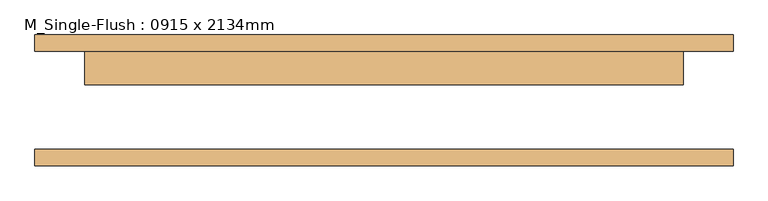
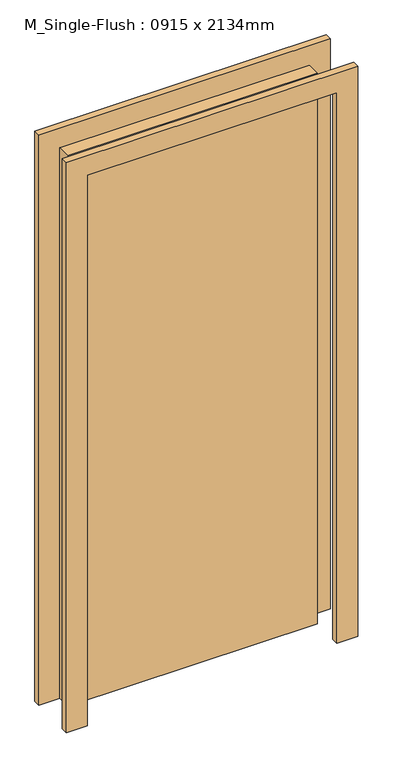
"""IFC4 building model written with IfcOpenShell, lengths in millimetres: door geometry, M_Single-Flush : 0915 x 2134mm."""

from ifc_helpers import new_model, si_unit, frame, origin, origin_with_axes, place, context, project, spatial, polyline, outline, extrude, source, transform, mapped, element, save


def m_single_flush_0915_x_2134mm_138fd904(model_context):
    return source(origin(), model_context, "Body", "SweptSolid", [
        extrude(outline(polyline([(2210.0, -533.5), (0.0, -533.5), (0.0, -457.5), (2134.0, -457.5), (2134.0, 457.5), (0.0, 457.5), (0.0, 533.5), (2210.0, 533.5), (2210.0, -533.5)])), frame((0.0, 75.0, 0.0), z_axis=(0.0, 1.0, 0.0), x_axis=(0.0, 0.0, 1.0)), (0.0, 0.0, 1.0), 25.0),
        extrude(outline(polyline([(2210.0, 533.5), (2210.0, -533.5), (0.0, -533.5), (0.0, -457.5), (2134.0, -457.5), (2134.0, 457.5), (0.0, 457.5), (0.0, 533.5), (2210.0, 533.5)])), frame((0.0, -100.0, 0.0), z_axis=(0.0, 1.0, 0.0), x_axis=(0.0, 0.0, 1.0)), (0.0, 0.0, 1.0), 25.0),
        extrude(outline(polyline([(457.5, 24.0), (-457.5, 24.0), (-457.5, 75.0), (457.5, 75.0), (457.5, 24.0)])), origin_with_axes(), (0.0, 0.0, 1.0), 2134.0),
    ])


if __name__ == "__main__":
    model = new_model("IFC4")
    model_context = context("Model", 3, world=origin())
    ifc_project = project(units=[si_unit("LENGTHUNIT", "METRE", prefix="MILLI")], contexts=[model_context])
    site = spatial("IfcSite", under=ifc_project)
    building = spatial("IfcBuilding", under=site)
    placement = place(None, origin())
    m_single_flush_0915_x_2134mm_shape = m_single_flush_0915_x_2134mm_138fd904(model_context)
    element("IfcDoor", 1, ObjectType="M_Single-Flush : 0915 x 2134mm", at=placement, inside=building, context=model_context, shape_type="MappedRepresentation", body=[
        mapped(m_single_flush_0915_x_2134mm_shape, transform((0.0, 0.0, 0.0), x_axis=(1.0, 0.0, 0.0), y_axis=(0.0, 1.0, 0.0), z_axis=(0.0, 0.0, 1.0))),
    ])
    save(model, "model.ifc")

# Revit data of these elements
# Type "M_Single-Flush : 0915 x 2134mm"
#   Type Mark = "15"
#   Thickness = 51 mm
#   Height = 2134 mm
#   Trim Projection Ext = 25 mm
#   Trim Projection Int = 25 mm
#   Trim Width = 76 mm
#   Width = 915 mm
#   Door Material = Door - Panel
#   Frame Material = Door - Frame
#   Function = (empty or 0)
#   Wall Closure = (empty or 0)
# Element 1 (IfcDoor, "M_Single-Flush : 0915 x 2134mm")
#   Materials on its faces: "Door - Frame", "Door - Panel"
# Materials
#   "Door - Panel": class "Wood", colour RGB 114 82 51, transparency 0
#   "Door - Frame": colour RGB 153 76 43, transparency 0
